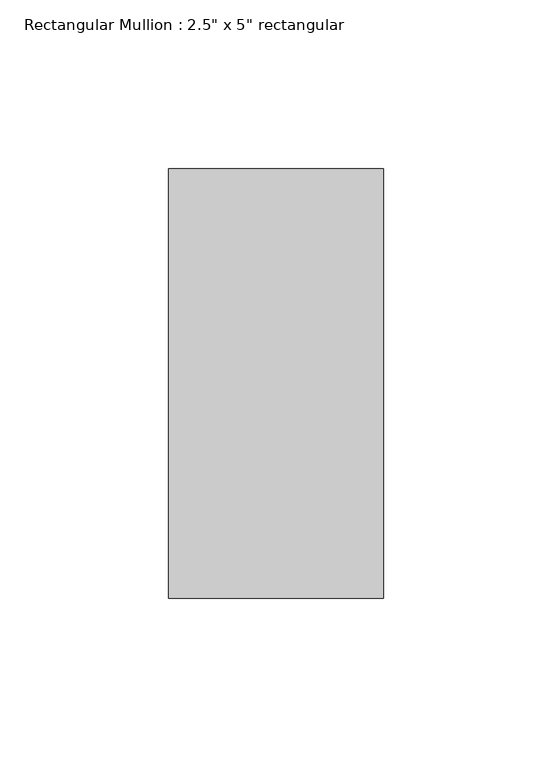
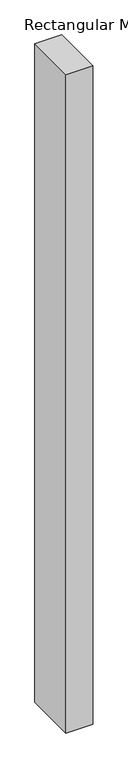
"""IFC4 building model written with IfcOpenShell, lengths in millimetres: member geometry."""

from ifc_helpers import new_model, si_unit, frame, origin, place, context, project, spatial, polyline, outline, extrude, source, transform, mapped, element, save


def member_72214107(model_context):
    return source(origin(), model_context, "Body", "SweptSolid", [
        extrude(outline(polyline([(31.75, 63.5), (31.75, -63.5), (-31.75, -63.5), (-31.75, 63.5), (31.75, 63.5)])), frame((0.0, 0.0, -1646.9365008), z_axis=(0.0, 0.0, 1.0), x_axis=(1.0, 0.0, 0.0)), (0.0, 0.0, 1.0), 1646.9365008),
    ])


if __name__ == "__main__":
    model = new_model("IFC4")
    model_context = context("Model", 3, world=origin())
    ifc_project = project(units=[si_unit("LENGTHUNIT", "METRE", prefix="MILLI")], contexts=[model_context])
    site = spatial("IfcSite", under=ifc_project)
    building = spatial("IfcBuilding", under=site)
    placement = place(None, origin())
    member_shape = member_72214107(model_context)
    element("IfcMember", 1, ObjectType="Rectangular Mullion : 2.5\" x 5\" rectangular", at=placement, inside=building, context=model_context, shape_type="MappedRepresentation", body=[
        mapped(member_shape, transform((0.0, 0.0, 0.0), x_axis=(1.0, 0.0, 0.0), y_axis=(0.0, 1.0, 0.0), z_axis=(0.0, 0.0, 1.0))),
    ])
    save(model, "model.ifc")

# Revit data of these elements
# Type "Rectangular Mullion : 2.5\" x 5\" rectangular"
#   built-in parameter 1007304 = 0.416667 (stored number, unit not read)
#   built-in parameter 1007301 = 0.104167 (stored number, unit not read)
#   built-in parameter 1007300 = 0.104167 (stored number, unit not read)
# Element 1 (IfcMember, "Rectangular Mullion : 2.5\" x 5\" rectangular")
#   Materials on its faces: "Aluminum"
# Materials
#   "Aluminum": class "Metal", colour RGB 247 247 247, transparency 0, Description = "Aluminum 6061", Cost = 0
